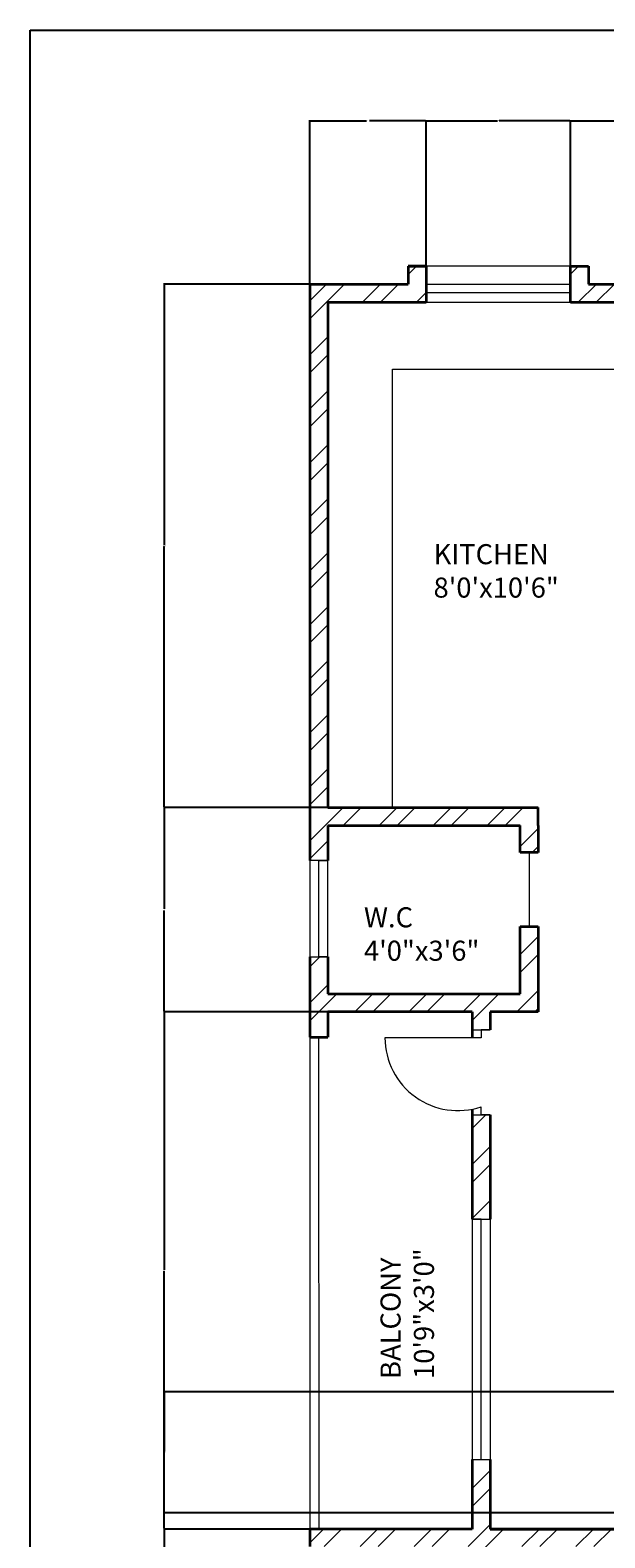
# Model space of a CAD drawing. Units: inches. Extents: x 1570 to 2186, y 1575 to 2421.
# Tile 6 of 10: x 1570 to 1713, y 2045 to 2421. Entities that reach past the tile are written whole.
import ezdxf

# ---------------------------------------------------------------- set-up
doc = ezdxf.new("R2010")
doc.units = ezdxf.units.IN
for name, color, linetype, lineweight in [('A-ANNO-DIMS', 2, 'Continuous', 18), ('A-ANNO-TTLB', 7, 'Continuous', 25), ('A-AREA-IDEN', 7, 'Continuous', 18), ('A-DOOR', 201, 'Continuous', 18), ('A-FLOR-CASE', 7, 'Continuous', 18), ('A-FLOR-HRAL', 201, 'Continuous', 18), ('A-GLAZ', 150, 'Continuous', 18), ('A-WALL', 7, 'Continuous', 35), ('A-WALL-PATT', 252, 'Continuous', 13)]:
    doc.layers.add(name, color=color, linetype=linetype, lineweight=lineweight)
doc.styles.get("Standard").update_dxf_attribs({"font": 'arial.ttf'})
doc.dimstyles.get("Standard").update_dxf_attribs({"dimtxt": 0.18, "dimasz": 0.18, "dimexe": 0.18, "dimexo": 0.0625, "dimgap": 0.09, "dimtad": 0, "dimtih": 1, "dimtoh": 1, "dimdec": 4, "dimzin": 0, "dimdsep": 46, "dimtxsty": 'Standard', "dimcen": 0.09, "dimadec": 0, "dimazin": 0, "dimtfac": 1, "dimtdec": 4, "dimtofl": 0, "dimtmove": 0, "dimatfit": 3, "dimfxl": 1, "dimtolj": 1, "dimtzin": 0, "dimarcsym": 0})

# ---------------------------------------------------------------- blocks, each defined once
blk = doc.blocks.new('*D22')
at = {"layer": 'A-ANNO-DIMS', "color": 0, "lineweight": -2, "transparency": 16777216}
for p, q in [((1639.59, 2357.71), (1639.59, 2398.63)), ((1639.77, 2398.45), (1653.71, 2398.45)), ((1668.44, 2398.45), (1654.5, 2398.45)), ((1668.62, 2362.21), (1668.62, 2398.63))]:
    blk.add_line(p, q, dxfattribs=at)
at = {"layer": 'A-ANNO-DIMS', "color": 0, "transparency": 16777216}
for points in [[(1639.77, 2398.48), (1639.77, 2398.42), (1639.59, 2398.45)], [(1668.44, 2398.48), (1668.44, 2398.42), (1668.62, 2398.45)]]:
    blk.add_solid(points, dxfattribs=at)
at = {"layer": 'Defpoints', "color": 0, "transparency": 16777216}
for p in [(1668.62, 2398.45), (1668.62, 2362.15), (1639.59, 2357.65)]:
    blk.add_point(p, dxfattribs=at)
at = {"layer": 'A-ANNO-DIMS', "color": 0, "transparency": 16777216, "insert": (1654.1, 2398.45), "char_height": 0.18, "attachment_point": 5}
blk.add_mtext('\\A1;29.03', dxfattribs=at)
blk = doc.blocks.new('*D23')
at = {"layer": 'A-ANNO-DIMS', "color": 0, "lineweight": -2, "transparency": 16777216}
for p, q in [((1668.62, 2362.21), (1668.62, 2398.63)), ((1668.8, 2398.45), (1686.4, 2398.45)), ((1704.44, 2398.45), (1686.84, 2398.45)), ((1704.62, 2362.21), (1704.62, 2398.63))]:
    blk.add_line(p, q, dxfattribs=at)
at = {"layer": 'A-ANNO-DIMS', "color": 0, "transparency": 16777216}
for points in [[(1668.8, 2398.48), (1668.8, 2398.42), (1668.62, 2398.45)], [(1704.44, 2398.48), (1704.44, 2398.42), (1704.62, 2398.45)]]:
    blk.add_solid(points, dxfattribs=at)
at = {"layer": 'Defpoints', "color": 0, "transparency": 16777216}
for p in [(1704.62, 2398.45), (1668.62, 2362.15), (1704.62, 2362.15)]:
    blk.add_point(p, dxfattribs=at)
at = {"layer": 'A-ANNO-DIMS', "color": 0, "transparency": 16777216, "insert": (1686.62, 2398.45), "char_height": 0.18, "attachment_point": 5}
blk.add_mtext('\\A1;36', dxfattribs=at)
blk = doc.blocks.new('*D24')
at = {"layer": 'A-ANNO-DIMS', "color": 0, "lineweight": -2, "transparency": 16777216}
for p, q in [((1704.62, 2362.21), (1704.62, 2398.63)), ((1704.8, 2398.45), (1732.96, 2398.45)), ((1761.92, 2398.45), (1733.75, 2398.45)), ((1762.1, 2362.21), (1762.1, 2398.63))]:
    blk.add_line(p, q, dxfattribs=at)
at = {"layer": 'A-ANNO-DIMS', "color": 0, "transparency": 16777216}
for points in [[(1704.8, 2398.48), (1704.8, 2398.42), (1704.62, 2398.45)], [(1761.92, 2398.48), (1761.92, 2398.42), (1762.1, 2398.45)]]:
    blk.add_solid(points, dxfattribs=at)
at = {"layer": 'Defpoints', "color": 0, "transparency": 16777216}
for p in [(1762.1, 2398.45), (1704.62, 2362.15), (1762.1, 2362.15)]:
    blk.add_point(p, dxfattribs=at)
at = {"layer": 'A-ANNO-DIMS', "color": 0, "transparency": 16777216, "insert": (1733.36, 2398.45), "char_height": 0.18, "attachment_point": 5}
blk.add_mtext('\\A1;57.48', dxfattribs=at)
blk = doc.blocks.new('*D35')
at = {"layer": 'A-ANNO-DIMS', "color": 0, "lineweight": -2, "transparency": 16777216}
for p, q in [((1639.53, 2047.15), (1603.11, 2047.15)), ((1603.29, 2046.97), (1603.29, 1980.63)), ((1603.29, 1913.93), (1603.29, 1980.27)), ((1639.53, 1913.75), (1603.11, 1913.75))]:
    blk.add_line(p, q, dxfattribs=at)
at = {"layer": 'A-ANNO-DIMS', "color": 0, "transparency": 16777216}
for points in [[(1603.26, 2046.97), (1603.32, 2046.97), (1603.29, 2047.15)], [(1603.26, 1913.93), (1603.32, 1913.93), (1603.29, 1913.75)]]:
    blk.add_solid(points, dxfattribs=at)
at = {"layer": 'Defpoints', "color": 0, "transparency": 16777216}
for p in [(1603.29, 2047.15), (1639.59, 2047.15), (1639.59, 1913.75)]:
    blk.add_point(p, dxfattribs=at)
at = {"layer": 'A-ANNO-DIMS', "color": 0, "transparency": 16777216, "insert": (1603.29, 1980.45), "char_height": 0.18, "attachment_point": 5}
blk.add_mtext('\\A1;133.4', dxfattribs=at)
blk = doc.blocks.new('*D36')
at = {"layer": 'A-ANNO-DIMS', "color": 0, "lineweight": -2, "transparency": 16777216}
for p, q in [((1644.03, 2176.15), (1603.11, 2176.15)), ((1603.29, 2175.97), (1603.29, 2111.83)), ((1603.29, 2047.33), (1603.29, 2111.47)), ((1639.53, 2047.15), (1603.11, 2047.15))]:
    blk.add_line(p, q, dxfattribs=at)
at = {"layer": 'A-ANNO-DIMS', "color": 0, "transparency": 16777216}
for points in [[(1603.26, 2175.97), (1603.32, 2175.97), (1603.29, 2176.15)], [(1603.26, 2047.33), (1603.32, 2047.33), (1603.29, 2047.15)]]:
    blk.add_solid(points, dxfattribs=at)
at = {"layer": 'Defpoints', "color": 0, "transparency": 16777216}
for p in [(1603.29, 2176.15), (1644.09, 2176.15), (1639.59, 2047.15)]:
    blk.add_point(p, dxfattribs=at)
at = {"layer": 'A-ANNO-DIMS', "color": 0, "transparency": 16777216, "insert": (1603.29, 2111.65), "char_height": 0.18, "attachment_point": 5}
blk.add_mtext('\\A1;129', dxfattribs=at)
blk = doc.blocks.new('*D37')
at = {"layer": 'A-ANNO-DIMS', "color": 0, "lineweight": -2, "transparency": 16777216}
for p, q in [((1644.03, 2227.15), (1603.11, 2227.15)), ((1603.29, 2226.97), (1603.29, 2201.83)), ((1603.29, 2176.33), (1603.29, 2201.47)), ((1644.03, 2176.15), (1603.11, 2176.15))]:
    blk.add_line(p, q, dxfattribs=at)
at = {"layer": 'A-ANNO-DIMS', "color": 0, "transparency": 16777216}
for points in [[(1603.26, 2226.97), (1603.32, 2226.97), (1603.29, 2227.15)], [(1603.26, 2176.33), (1603.32, 2176.33), (1603.29, 2176.15)]]:
    blk.add_solid(points, dxfattribs=at)
at = {"layer": 'Defpoints', "color": 0, "transparency": 16777216}
for p in [(1603.29, 2227.15), (1644.09, 2227.15), (1644.09, 2176.15)]:
    blk.add_point(p, dxfattribs=at)
at = {"layer": 'A-ANNO-DIMS', "color": 0, "transparency": 16777216, "insert": (1603.29, 2201.65), "char_height": 0.18, "attachment_point": 5}
blk.add_mtext('\\A1;51', dxfattribs=at)
blk = doc.blocks.new('*D38')
at = {"layer": 'A-ANNO-DIMS', "color": 0, "lineweight": -2, "transparency": 16777216}
for p, q in [((1639.53, 2357.65), (1603.11, 2357.65)), ((1603.29, 2357.47), (1603.29, 2292.58)), ((1603.29, 2227.33), (1603.29, 2292.22)), ((1644.03, 2227.15), (1603.11, 2227.15))]:
    blk.add_line(p, q, dxfattribs=at)
at = {"layer": 'A-ANNO-DIMS', "color": 0, "transparency": 16777216}
for points in [[(1603.26, 2357.47), (1603.32, 2357.47), (1603.29, 2357.65)], [(1603.26, 2227.33), (1603.32, 2227.33), (1603.29, 2227.15)]]:
    blk.add_solid(points, dxfattribs=at)
at = {"layer": 'Defpoints', "color": 0, "transparency": 16777216}
for p in [(1603.29, 2357.65), (1639.59, 2357.65), (1644.09, 2227.15)]:
    blk.add_point(p, dxfattribs=at)
at = {"layer": 'A-ANNO-DIMS', "color": 0, "transparency": 16777216, "insert": (1603.29, 2292.4), "char_height": 0.18, "attachment_point": 5}
blk.add_mtext('\\A1;130.5', dxfattribs=at)
blk = doc.blocks.new('*D42')
at = {"layer": 'A-ANNO-DIMS', "color": 0, "lineweight": -2, "transparency": 16777216}
for p, q in [((1913.53, 2081.37), (1603.11, 2081.37)), ((1603.29, 2081.19), (1603.29, 2066.47)), ((1603.29, 2051.39), (1603.29, 2066.11)), ((1913.53, 2051.21), (1603.11, 2051.21))]:
    blk.add_line(p, q, dxfattribs=at)
at = {"layer": 'A-ANNO-DIMS', "color": 0, "transparency": 16777216}
for points in [[(1603.26, 2081.19), (1603.32, 2081.19), (1603.29, 2081.37)], [(1603.26, 2051.39), (1603.32, 2051.39), (1603.29, 2051.21)]]:
    blk.add_solid(points, dxfattribs=at)
at = {"layer": 'Defpoints', "color": 0, "transparency": 16777216}
for p in [(1603.29, 2081.37), (1913.59, 2081.37), (1913.59, 2051.21)]:
    blk.add_point(p, dxfattribs=at)
at = {"layer": 'A-ANNO-DIMS', "color": 0, "transparency": 16777216, "insert": (1603.29, 2066.29), "char_height": 0.18, "attachment_point": 5}
blk.add_mtext('\\A1;30.165', dxfattribs=at)

msp = doc.modelspace()

# ---------------------------------------------------------------- hatches: boundary and pattern name
at = {"layer": 'A-WALL-PATT'}
h = msp.add_hatch(dxfattribs=at)
h.set_pattern_fill('ANSI32', color=256)
h.paths.add_polyline_path([(1762.0975, 2362.1492), (1757.5975, 2362.1492), (1757.5975, 2357.6492), (1709.1163, 2357.6492), (1709.1163, 2362.1492), (1704.6163, 2362.1492), (1704.6163, 2353.1492), (1740.0886, 2353.1492), (1740.0886, 2261.8115), (1744.5886, 2261.8115), (1744.5886, 2353.1492), (1762.0975, 2353.1492)])
h.paths.add_polyline_path([(1890.2592, 2362.1492), (1885.7592, 2362.1492), (1826.5975, 2362.1492), (1822.0975, 2362.1492), (1822.0975, 2353.1492), (1862.5886, 2353.1492), (1862.5886, 2227.1492), (1744.5886, 2227.1492), (1744.5886, 2229.5389), (1742.3386, 2229.5389), (1740.0886, 2229.5389), (1740.0886, 2222.6492), (1744.5886, 2222.6492), (1756.186, 2222.6492), (1756.186, 2216.3571), (1760.686, 2216.3571), (1760.686, 2222.6492), (1832.686, 2222.6492), (1832.686, 2212.5994), (1837.186, 2212.5994), (1837.186, 2222.6492), (1893.186, 2222.6492), (1893.186, 2212.5994), (1897.686, 2212.5994), (1897.686, 2222.6492), (1989.5886, 2222.6492), (1989.5886, 2227.1492), (1989.5886, 2232.6585), (1987.3386, 2232.6585), (1985.0886, 2232.6585), (1985.0886, 2227.1492), (1867.0886, 2227.1492), (1867.0886, 2353.1492), (1890.2592, 2353.1492)])
h.paths.add_polyline_path([(1644.0886, 2353.1492), (1668.6163, 2353.1492), (1668.6163, 2362.1492), (1664.1163, 2362.1492), (1664.1163, 2358.9932), (1664.1163, 2357.6492), (1639.5886, 2357.6492), (1639.5886, 2213.8746), (1644.0886, 2213.8746), (1644.0886, 2222.6492), (1692.0886, 2222.6492), (1692.0886, 2215.9343), (1696.5886, 2215.9343), (1696.5886, 2222.6492), (1696.5886, 2227.1492), (1644.0886, 2227.1492)])
h.paths.add_polyline_path([(2013.0435, 2362.1492), (2008.5435, 2362.1492), (2008.5435, 2357.6492), (1954.7592, 2357.6492), (1954.7592, 2362.1492), (1950.2592, 2362.1492), (1950.2592, 2353.1492), (1985.0886, 2353.1492), (1985.0886, 2260.8534), (1989.5886, 2260.8534), (1989.5886, 2353.1492), (2013.0435, 2353.1492)])
h.paths.add_polyline_path([(2090.0886, 2357.6492), (2053.5435, 2357.6492), (2053.5435, 2362.1492), (2049.0435, 2362.1492), (2049.0435, 2353.1492), (2085.5886, 2353.1492), (2085.5886, 2227.1492), (2033.0886, 2227.1492), (2033.0886, 2222.6492), (2033.0886, 2214.4464), (2037.5886, 2214.4464), (2037.5886, 2222.6492), (2085.5886, 2222.6492), (2085.5886, 2212.4409), (2090.0886, 2212.4409)])
h.paths.add_polyline_path([(2090.0886, 2188.4409), (2087.8386, 2188.4409), (2085.5886, 2188.4409), (2085.5886, 2180.6492), (2037.5886, 2180.6492), (2037.5886, 2196.7956), (2033.0886, 2196.7956), (2033.0886, 2176.1492), (2037.5886, 2176.1492), (2045.0886, 2176.1492), (2045.0886, 2169.8988), (2049.5886, 2169.8988), (2049.5886, 2176.1492), (2085.5886, 2176.1492), (2085.5886, 2167.785), (2090.0886, 2167.785)])
h.paths.add_polyline_path([(2049.5886, 2147.4502), (2047.3386, 2147.4502), (2045.0886, 2147.4502), (2045.0886, 2124.4703), (2049.5886, 2124.4703)])
h.paths.add_polyline_path([(2090.0886, 2047.1492), (2049.5886, 2047.1492), (2049.5886, 2064.4703), (2045.0886, 2064.4703), (2045.0886, 2047.1492), (1918.0886, 2047.1492), (1918.0886, 2051.2061), (1913.5886, 2051.2061), (1913.5886, 2047.1492), (1913.5886, 2036.6872), (1918.0886, 2036.6872), (1918.0886, 2042.7492), (2045.0886, 2042.7492), (2045.0886, 2027.0686), (2049.5886, 2027.0686), (2049.5886, 2042.7492), (2090.0886, 2042.7492)])
h.paths.add_polyline_path([(1918.0886, 2005.9338), (1915.8386, 2005.9338), (1913.5886, 2005.9338), (1913.5886, 1913.7492), (1918.0886, 1913.7492)])
h.paths.add_polyline_path([(2090.0886, 1913.7492), (2049.5886, 1913.7492), (2045.0886, 1913.7492), (2033.0886, 1913.7492), (2033.0886, 1909.2492), (2033.0886, 1900.9803), (2037.5886, 1900.9803), (2037.5886, 1909.2492), (2085.5886, 1909.2492), (2085.5886, 1861.2492), (2037.5886, 1861.2492), (2037.5886, 1880.0859), (2033.0886, 1880.0859), (2033.0886, 1856.7492), (2085.5886, 1856.7492), (2085.5886, 1730.7492), (2054.2483, 1730.7492), (2054.2483, 1721.7492), (2058.7483, 1721.7492), (2058.7483, 1726.2492), (2090.0886, 1726.2492)])
h.paths.add_polyline_path([(2049.5886, 1967.0686), (2045.0886, 1967.0686), (2045.0886, 1913.7492), (2049.5886, 1913.7492)])
h.paths.add_polyline_path([(1989.5886, 1824.1695), (1987.3386, 1824.1695), (1985.0886, 1824.1695), (1985.0886, 1730.7492), (1989.5886, 1730.7492)])
h.paths.add_polyline_path([(1989.5886, 1861.2492), (1974.9963, 1861.2492), (1974.9963, 1865.9306), (1972.7463, 1865.9306), (1970.4963, 1865.9306), (1970.4963, 1861.2492), (1898.4963, 1861.2492), (1898.4963, 1874.2999), (1893.9963, 1874.2999), (1893.9963, 1861.2492), (1890.5886, 1861.2492), (1837.9963, 1861.2492), (1837.9963, 1874.3159), (1833.4963, 1874.3159), (1833.4963, 1861.2492), (1761.4963, 1861.2492), (1761.4963, 1865.0209), (1759.2463, 1865.0209), (1756.9963, 1865.0209), (1756.9963, 1861.2492), (1740.0886, 1861.2492), (1740.0886, 1856.7492), (1740.0886, 1850.7206), (1744.5886, 1850.7206), (1744.5886, 1856.7492), (1985.0886, 1856.7492), (1985.0886, 1851.0804), (1989.5886, 1851.0804), (1989.5886, 1856.7492)])
h.paths.add_polyline_path([(1989.5886, 1913.7492), (1740.0886, 1913.7492), (1740.0886, 1909.2492), (1756.9963, 1909.2492), (1756.9963, 1890.279), (1761.4963, 1890.279), (1761.4963, 1909.2492), (1833.4963, 1909.2492), (1833.4963, 1898.3159), (1837.9963, 1898.3159), (1837.9963, 1909.2492), (1890.5886, 1909.2492), (1893.9963, 1909.2492), (1893.9963, 1898.2999), (1898.4963, 1898.2999), (1898.4963, 1909.2492), (1970.4963, 1909.2492), (1970.4963, 1886.9887), (1974.9963, 1886.9887), (1974.9963, 1909.2492), (1989.5886, 1909.2492)])
h.paths.add_polyline_path([(1893.7344, 1730.7492), (1867.0886, 1730.7492), (1867.0886, 1856.7492), (1862.5886, 1856.7492), (1862.5886, 1730.7492), (1824.0492, 1730.7492), (1824.0492, 1721.7492), (1893.7344, 1721.7492)])
h.paths.add_polyline_path([(2018.2483, 1730.7492), (1953.7344, 1730.7492), (1953.7344, 1721.7492), (1958.2344, 1721.7492), (1958.2344, 1726.2492), (2013.7483, 1726.2492), (2013.7483, 1721.7492), (2018.2483, 1721.7492)])
h.paths.add_polyline_path([(1768.5492, 1730.7492), (1764.0492, 1730.7492), (1744.5886, 1730.7492), (1744.5886, 1819.4364), (1742.3386, 1819.4364), (1740.0886, 1819.4364), (1740.0886, 1730.7492), (1697.3801, 1730.7492), (1697.3801, 1721.7492), (1701.8801, 1721.7492), (1701.8801, 1726.2492), (1764.0492, 1726.2492), (1764.0492, 1721.7492), (1768.5492, 1721.7492)])
h.paths.add_polyline_path([(1644.0886, 1856.7492), (1639.5886, 1856.7492), (1639.5886, 1726.2492), (1657.0315, 1726.2492), (1657.0315, 1721.7492), (1661.3801, 1721.7492), (1661.3801, 1730.7492), (1644.0886, 1730.7492)])
h.paths.add_polyline_path([(1696.5886, 1876.1809), (1692.0886, 1876.1809), (1692.0886, 1861.2492), (1684.5886, 1861.2492), (1644.0886, 1861.2492), (1644.0886, 1909.2492), (1692.0886, 1909.2492), (1692.0886, 1900.3394), (1696.5886, 1900.3394), (1696.5886, 1913.7492), (1684.5886, 1913.7492), (1684.5886, 1920.2115), (1682.3386, 1920.2115), (1680.0886, 1920.2115), (1680.0886, 1913.7492), (1639.5886, 1913.7492), (1639.5886, 1856.7492), (1684.5886, 1856.7492), (1692.0886, 1856.7492), (1696.5886, 1856.7492)])
h.paths.add_polyline_path([(1684.5886, 2042.7492), (1811.5886, 2042.7492), (1811.5886, 2038.2991), (1816.0886, 2038.2991), (1816.0886, 2042.7492), (1816.0886, 2052.5708), (1813.8386, 2052.5708), (1811.5886, 2052.5708), (1811.5886, 2047.1492), (1684.5886, 2047.1492), (1684.5886, 2064.4703), (1680.0886, 2064.4703), (1680.0886, 2047.1492), (1639.5886, 2047.1492), (1639.5886, 2042.7492), (1680.0886, 2042.7492), (1680.0886, 2024.0762), (1684.5886, 2024.0762)])
h.paths.add_polyline_path([(1684.5886, 1964.0762), (1680.0886, 1964.0762), (1680.0886, 1944.6145), (1684.5886, 1944.6145)])
h.paths.add_polyline_path([(1816.0886, 1973.7492), (1876.0886, 1973.7492), (1876.0886, 1959.17), (1880.5886, 1959.17), (1880.5886, 1973.7492), (1880.5886, 1978.2492), (1816.0886, 1978.2492), (1816.0886, 2005.9338), (1813.8386, 2005.9338), (1811.5886, 2005.9338), (1811.5886, 1913.7492), (1816.0886, 1913.7492)])
h.paths.add_polyline_path([(1837.186, 2180.6492), (1837.186, 2188.5994), (1834.936, 2188.5994), (1832.686, 2188.5994), (1832.686, 2180.6492), (1760.686, 2180.6492), (1760.686, 2197.4807), (1756.186, 2197.4807), (1756.186, 2180.6492), (1744.5886, 2180.6492), (1740.0886, 2180.6492), (1740.0886, 2176.1492), (1837.186, 2176.1492)])
h.paths.add_polyline_path([(1974.186, 2196.8744), (1971.936, 2196.8744), (1969.686, 2196.8744), (1969.686, 2180.6492), (1897.686, 2180.6492), (1897.686, 2188.5994), (1895.436, 2188.5994), (1893.186, 2188.5994), (1893.186, 2180.6492), (1893.186, 2176.1492), (1974.186, 2176.1492)])
h.paths.add_polyline_path([(1918.0886, 2176.1492), (1913.5886, 2176.1492), (1913.5886, 2081.3709), (1918.0886, 2081.3709)])
h.paths.add_polyline_path([(1816.0886, 2176.1492), (1811.5886, 2176.1492), (1811.5886, 2081.3709), (1816.0886, 2081.3709)])
h.paths.add_polyline_path([(1684.5886, 2150.4939), (1682.3386, 2150.4939), (1680.0886, 2150.4939), (1680.0886, 2124.4703), (1684.5886, 2124.4703)])
h.paths.add_polyline_path([(1696.5886, 2180.6492), (1696.5886, 2197.4701), (1692.0886, 2197.4701), (1692.0886, 2180.6492), (1644.0886, 2180.6492), (1644.0886, 2189.8746), (1641.8386, 2189.8746), (1639.5886, 2189.8746), (1639.5886, 2169.814), (1644.0886, 2169.814), (1644.0886, 2176.1492), (1680.0886, 2176.1492), (1680.0886, 2171.7002), (1684.5886, 2171.7002), (1684.5886, 2176.1492), (1696.5886, 2176.1492)])

# ---------------------------------------------------------------- linework, layer by layer
at = {"layer": 'A-ANNO-TTLB'}
msp.add_lwpolyline([(1569.8198, 2421.0436), (2186.3437, 2421.0436), (2186.3437, 1574.5084), (1569.8198, 1574.5084)], close=True, dxfattribs=at)
at = {"layer": 'A-DOOR'}
for p, q in [((1694.3386, 2215.9343), (1694.3386, 2197.4701)), ((1680.0886, 2171.7002), (1684.5886, 2171.7002)), ((1684.5886, 2171.7002), (1682.3386, 2171.7002)), ((1682.3386, 2171.7002), (1682.3386, 2169.7002)), ((1682.3386, 2169.7002), (1658.3386, 2169.7002)), ((1682.3386, 2150.4939), (1682.3386, 2152.4939)), ((1680.0886, 2150.4939), (1684.5886, 2150.4939)), ((1684.5886, 2150.4939), (1682.3386, 2150.4939))]:
    msp.add_line(p, q, dxfattribs=at)
msp.add_arc((1676.5065, 2169.7002), 18.1679, 180, 288.724201, dxfattribs=at)
at = {"layer": 'A-FLOR-CASE'}
for p, q in [((1660.2219, 2227.1492), (1660.2219, 2336.4511)), ((1660.2219, 2336.4511), (1740.0886, 2336.4511))]:
    msp.add_line(p, q, dxfattribs=at)
at = {"layer": 'A-FLOR-HRAL'}
for p, q in [((1639.5886, 2169.814), (1639.5886, 2047.1492)), ((1641.9256, 2047.1492), (1641.8386, 2169.814))]:
    msp.add_line(p, q, dxfattribs=at)
at = {"layer": 'A-GLAZ'}
for p, q in [((1704.6163, 2362.1492), (1668.6163, 2362.1492)), ((1668.6163, 2357.6492), (1704.6163, 2357.6492)), ((1668.6163, 2355.5993), (1704.6163, 2355.5993)), ((1668.6163, 2353.1492), (1704.6163, 2353.1492)), ((1644.0886, 2213.8746), (1639.5886, 2213.8746)), ((1639.5886, 2213.8746), (1639.5886, 2189.8746)), ((1641.8386, 2189.8746), (1641.8386, 2213.8746)), ((1641.8386, 2213.8746), (1644.0886, 2213.8746)), ((1644.0886, 2189.8746), (1644.0886, 2213.8746)), ((1639.5886, 2189.8746), (1644.0886, 2189.8746)), ((1644.0886, 2189.8746), (1641.8386, 2189.8746)), ((1682.3386, 2124.4703), (1680.0886, 2124.4703)), ((1680.0886, 2124.4703), (1684.5886, 2124.4703)), ((1680.0886, 2124.4703), (1680.0886, 2064.4703)), ((1682.3386, 2064.4703), (1682.3386, 2124.4703)), ((1684.5886, 2124.4703), (1684.5886, 2064.4703)), ((1680.0886, 2064.4703), (1684.5886, 2064.4703))]:
    msp.add_line(p, q, dxfattribs=at)
at = {"layer": 'A-WALL'}
for p, q in [((1664.1163, 2362.1492), (1668.6163, 2362.1492)), ((1668.6163, 2362.1492), (1664.1163, 2362.1492)), ((1664.1163, 2362.1492), (1664.1163, 2358.9932)), ((1668.6163, 2362.1492), (1668.6163, 2353.1492)), ((1704.6163, 2353.1492), (1704.6163, 2362.1492)), ((1704.6163, 2362.1492), (1709.1163, 2362.1492)), ((1704.6163, 2362.1492), (1709.1163, 2362.1492)), ((1709.1163, 2362.1492), (1709.1163, 2357.6492)), ((1664.1163, 2358.9932), (1664.1163, 2357.6492)), ((1639.5886, 2357.6492), (1664.1163, 2357.6492)), ((1639.5886, 2357.6492), (1639.5886, 2213.8746)), ((1709.1163, 2357.6492), (1757.5975, 2357.6492)), ((1644.0886, 2353.1492), (1668.6163, 2353.1492)), ((1644.0886, 2353.1492), (1644.0886, 2227.1492)), ((1704.6163, 2353.1492), (1740.0886, 2353.1492)), ((1644.0886, 2227.1492), (1696.5886, 2227.1492)), ((1696.5886, 2222.6492), (1696.5886, 2227.1492)), ((1644.0886, 2222.6492), (1692.0886, 2222.6492)), ((1644.0886, 2222.6492), (1644.0886, 2213.8746)), ((1692.0886, 2215.9343), (1692.0886, 2222.6492)), ((1696.5886, 2222.6492), (1696.5886, 2215.9343)), ((1696.5886, 2215.9343), (1692.0886, 2215.9343)), ((1692.0886, 2180.6492), (1692.0886, 2197.4701)), ((1692.0886, 2197.4701), (1696.5886, 2197.4701)), ((1696.5886, 2197.4701), (1696.5886, 2180.6492)), ((1639.5886, 2189.8746), (1639.5886, 2169.814)), ((1644.0886, 2189.8746), (1644.0886, 2180.6492)), ((1644.0886, 2180.6492), (1692.0886, 2180.6492)), ((1696.5886, 2180.6492), (1696.5886, 2176.1492)), ((1644.0886, 2176.1492), (1644.0886, 2169.814)), ((1680.0886, 2176.1492), (1644.0886, 2176.1492)), ((1680.0886, 2176.1492), (1680.0886, 2169.7002)), ((1696.5886, 2176.1492), (1684.5886, 2176.1492)), ((1684.5886, 2176.1492), (1684.5886, 2171.7002)), ((1639.5886, 2169.814), (1644.0886, 2169.814)), ((1680.0886, 2151.889), (1680.0886, 2124.4703)), ((1684.5886, 2150.4939), (1684.5886, 2124.4703)), ((1680.0886, 2064.4703), (1680.0886, 2047.1492)), ((1684.5886, 2064.4703), (1684.5886, 2047.1492)), ((1639.5886, 2047.1492), (1639.5886, 2042.7492)), ((1680.0886, 2047.1492), (1639.5886, 2047.1492)), ((1684.5886, 2047.1492), (1811.5886, 2047.1492)), ((1811.5886, 2047.1492), (1684.5886, 2047.1492))]:
    msp.add_line(p, q, dxfattribs=at)

# ---------------------------------------------------------------- texts
at = {"layer": 'A-AREA-IDEN', "char_height": 5, "attachment_point": 1}
for s, width, insert in [('KITCHEN\\P8\'0\'x10\'6"', 156.004348, (1670.4581, 2292.8279)), ('W.C \\P4\'0"x3\'6"', 85.755775, (1653.0959, 2202.2409))]:
    msp.add_mtext_dynamic_manual_height_columns(s, width=width, gutter_width=12.5, heights=[0], dxfattribs=dict(at, insert=insert))
at = {"layer": 'A-AREA-IDEN', "insert": (1657.2228, 2084.5832), "char_height": 5, "attachment_point": 1, "rotation": 90}
msp.add_mtext_dynamic_manual_height_columns('BALCONY\\P10\'9"x3\'0"', width=184.453403, gutter_width=12.5, heights=[0], dxfattribs=at)

# ---------------------------------------------------------------- dimensions: what is measured, and where the dimension line sits
at = {"layer": 'A-ANNO-DIMS'}
for base, p1, p2, override, picture, middle in [((1668.6163, 2398.4492), (1639.5886, 2357.6492), (1668.6163, 2362.1492), {"dimdec": 2, "dimlfac": 1, "dimrnd": 0, "dimzin": 0, "dimdsep": 46, "dimlunit": 2}, '*D22', (1654.1025, 2398.4492)), ((1704.6163, 2398.4492), (1668.6163, 2362.1492), (1704.6163, 2362.1492), {"dimdec": 0, "dimlfac": 1, "dimrnd": 0, "dimzin": 0, "dimdsep": 46, "dimlunit": 2}, '*D23', (1686.6163, 2398.4492)), ((1762.0975, 2398.4492), (1704.6163, 2362.1492), (1762.0975, 2362.1492), {"dimdec": 2, "dimlfac": 1, "dimrnd": 0, "dimzin": 0, "dimdsep": 46, "dimlunit": 2}, '*D24', (1733.3569, 2398.4492))]:
    dim = msp.add_linear_dim(base=base, p1=p1, p2=p2, dimstyle='Standard', override=override, dxfattribs=at)
    dim.commit()
    dim.dimension.update_dxf_attribs({"geometry": picture, "text_midpoint": middle})
for base, p1, p2, override, picture, middle in [((1603.2886, 2357.6492), (1644.0886, 2227.1492), (1639.5886, 2357.6492), {"dimdec": 1, "dimlfac": 1, "dimrnd": 0, "dimzin": 0, "dimdsep": 46, "dimlunit": 2}, '*D38', (1603.2886, 2292.3992)), ((1603.2886, 2227.1492), (1644.0886, 2176.1492), (1644.0886, 2227.1492), {"dimdec": 0, "dimlfac": 1, "dimrnd": 0, "dimzin": 0, "dimdsep": 46, "dimlunit": 2}, '*D37', (1603.2886, 2201.6492)), ((1603.2886, 2176.1492), (1639.5886, 2047.1492), (1644.0886, 2176.1492), {"dimdec": 0, "dimlfac": 1, "dimrnd": 0, "dimzin": 0, "dimdsep": 46, "dimlunit": 2}, '*D36', (1603.2886, 2111.6492)), ((1603.2886, 2081.3709), (1913.5886, 2051.2061), (1913.5886, 2081.3709), {"dimdec": 3, "dimlfac": 1, "dimrnd": 0, "dimzin": 0, "dimdsep": 46, "dimlunit": 2}, '*D42', (1603.2886, 2066.2885)), ((1603.2886, 2047.1492), (1639.5886, 1913.7492), (1639.5886, 2047.1492), {"dimdec": 1, "dimlfac": 1, "dimrnd": 0, "dimzin": 0, "dimdsep": 46, "dimlunit": 2}, '*D35', (1603.2886, 1980.4492))]:
    dim = msp.add_linear_dim(base=base, p1=p1, p2=p2, angle=90, dimstyle='Standard', override=override, dxfattribs=at)
    dim.commit()
    dim.dimension.update_dxf_attribs({"geometry": picture, "text_midpoint": middle})

doc.saveas('drawing.dxf')
